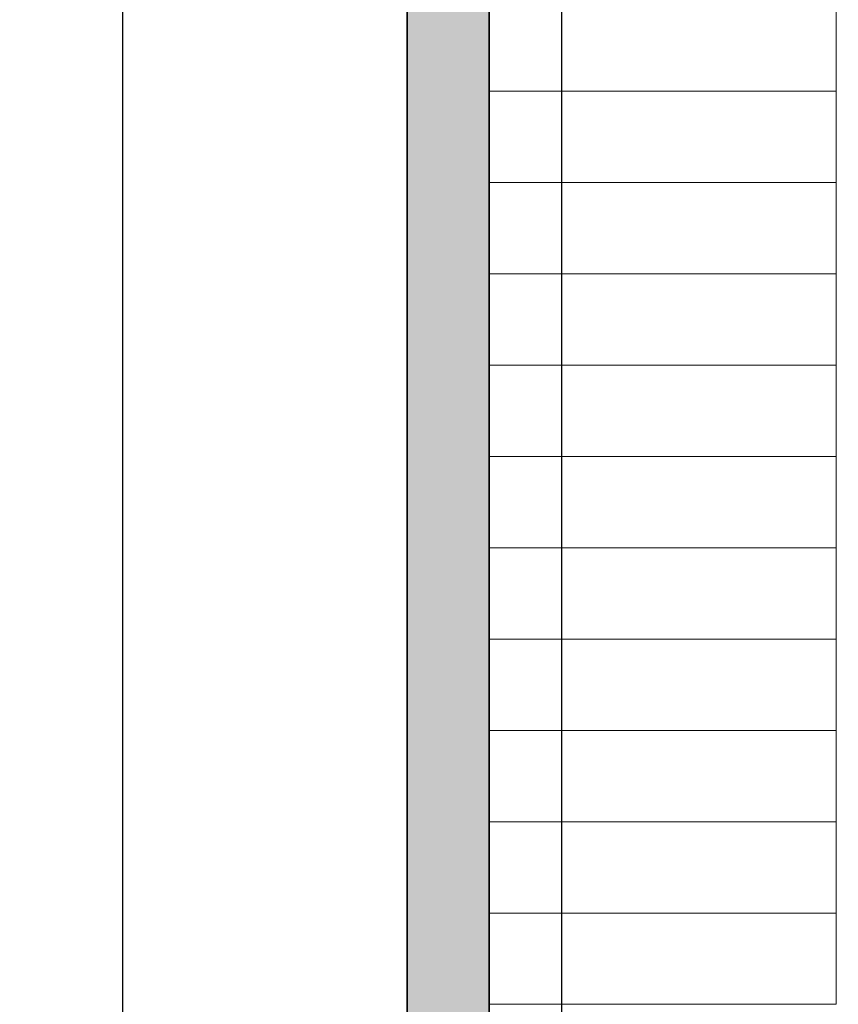
# Model space of a CAD drawing. Units: inches. Extents: x 37 to 706, y -568 to 110.
# Tile 2 of 24: x 37 to 126, y -450 to -342. Entities that reach past the tile are written whole.
import ezdxf

# ---------------------------------------------------------------- set-up
doc = ezdxf.new("R2010")
doc.units = ezdxf.units.IN
doc.header["$MEASUREMENT"] = 0
for name, color, linetype, lineweight in [('A-ANNO-DIMS', 2, 'Continuous', 18), ('A-FLOR-STRS', 7, 'Continuous', 18), ('A-WALL', 7, 'Continuous', 35), ('A-WALL-PATT', 252, 'Continuous', 13)]:
    doc.layers.add(name, color=color, linetype=linetype, lineweight=lineweight)
doc.styles.get("Standard").update_dxf_attribs({"font": 'arial.ttf'})
doc.dimstyles.get("Standard").update_dxf_attribs({"dimtxt": 0.18, "dimasz": 0.18, "dimexe": 0.18, "dimexo": 0.0625, "dimgap": 0.09, "dimtad": 0, "dimtih": 1, "dimtoh": 1, "dimdec": 0, "dimzin": 0, "dimdsep": 46, "dimlunit": 3, "dimtxsty": 'Standard', "dimcen": 0.09, "dimadec": 0, "dimazin": 0, "dimtfac": 1, "dimtdec": 0, "dimtofl": 0, "dimtmove": 0, "dimatfit": 3, "dimfxl": 1, "dimtolj": 1, "dimtzin": 0, "dimarcsym": 0})

# ---------------------------------------------------------------- blocks, each defined once
blk = doc.blocks.new('*D3')
at = {"layer": 'A-ANNO-DIMS', "color": 0, "lineweight": -2, "transparency": 16777216}
for p, q in [((78.9, 51.29), (47.67, 51.29)), ((47.85, 51.11), (47.85, -228.11)), ((47.85, -513.53), (47.85, -234.31)), ((78.9, -513.71), (47.67, -513.71))]:
    blk.add_line(p, q, dxfattribs=at)
at = {"layer": 'A-ANNO-DIMS', "color": 0, "transparency": 16777216}
for points in [[(47.82, 51.11), (47.88, 51.11), (47.85, 51.29)], [(47.82, -513.53), (47.88, -513.53), (47.85, -513.71)]]:
    blk.add_solid(points, dxfattribs=at)
at = {"layer": 'Defpoints', "color": 0, "transparency": 16777216}
for p in [(78.96, 51.29), (47.85, -513.71), (78.96, -513.71)]:
    blk.add_point(p, dxfattribs=at)
at = {"layer": 'A-ANNO-DIMS', "color": 0, "transparency": 16777216, "insert": (47.85, -231.21), "char_height": 6, "attachment_point": 5}
blk.add_mtext('\\A1;47\'-1"', dxfattribs=at)
blk = doc.blocks.new('*D54')
at = {"layer": 'A-ANNO-DIMS', "color": 0, "lineweight": -2, "transparency": 16777216}
for p, q in [((87.96, -303.77), (87.96, -567.64)), ((95.87, -303.77), (95.87, -567.64)), ((88.14, -567.46), (91.59, -567.46)), ((95.69, -567.46), (92.24, -567.46))]:
    blk.add_line(p, q, dxfattribs=at)
at = {"layer": 'A-ANNO-DIMS', "color": 0, "transparency": 16777216}
for points in [[(88.14, -567.43), (88.14, -567.49), (87.96, -567.46)], [(95.69, -567.43), (95.69, -567.49), (95.87, -567.46)]]:
    blk.add_solid(points, dxfattribs=at)
at = {"layer": 'Defpoints', "color": 0, "transparency": 16777216}
for p in [(87.96, -303.71), (95.87, -303.71), (95.87, -567.46)]:
    blk.add_point(p, dxfattribs=at)
at = {"layer": 'A-ANNO-DIMS', "color": 0, "transparency": 16777216, "insert": (91.91, -567.46), "char_height": 0.18, "attachment_point": 5}
blk.add_mtext('\\A1;0\'-8"', dxfattribs=at)

msp = doc.modelspace()

# ---------------------------------------------------------------- hatches: boundary and pattern name
at = {"layer": 'A-WALL-PATT'}
h = msp.add_hatch(color=256, dxfattribs=at)
h.dxf.hatch_style = 1
h.paths.add_polyline_path([(220.96, -351.71), (211.96, -351.71), (211.96, -513.71), (254.96, -513.71), (254.96, -504.71), (220.96, -504.71)], flags=17)
h.paths.add_polyline_path([(220.96, -294.71), (211.96, -294.71), (211.96, -303.71), (220.96, -303.71)], flags=17)
h.paths.add_polyline_path([(175.96, -294.71), (155.87, -294.71), (155.87, -303.71), (155.96, -303.71), (175.96, -303.71)], flags=17)
h.paths.add_polyline_path([(220.96, -16.71), (211.96, -16.71), (211.96, -142.71), (220.96, -142.71)], flags=17)
h.paths.add_polyline_path([(357.96, 51.29), (78.96, 51.29), (78.96, -513.71), (87.96, -513.71), (87.96, -303.71), (95.87, -303.71), (95.87, -294.71), (87.96, -294.71), (87.96, -142.71), (187.96, -142.71), (187.96, -133.71), (87.96, -133.71), (87.96, -25.71), (106.96, -25.71), (106.96, -16.71), (87.96, -16.71), (87.96, 42.29), (348.96, 42.29), (348.96, 17.13), (348.96, -133.71), (246.96, -133.71), (246.96, -142.71), (348.96, -142.71), (348.96, -294.71), (251.96, -294.71), (251.96, -303.71), (348.96, -303.71), (348.96, -351.71), (260.96, -351.71), (260.96, -329.71), (251.96, -329.71), (251.96, -360.71), (327.45, -360.71), (348.96, -360.71), (348.96, -504.71), (314.96, -504.71), (314.96, -513.71), (357.96, -513.71)])
h.paths.add_polyline_path([(416.96, -303.71), (402.96, -303.71), (402.96, -151.71), (478.96, -151.71), (478.96, -142.71), (402.96, -142.71), (402.96, -22.71), (409.96, -22.71), (409.96, -13.71), (402.96, -13.71), (402.96, 42.29), (663.96, 42.29), (663.96, -303.71), (566.96, -303.71), (566.96, -312.71), (663.96, -312.71), (663.96, -360.71), (575.96, -360.71), (575.96, -338.71), (566.96, -338.71), (566.96, -360.71), (566.96, -369.71), (642.45, -369.71), (663.96, -369.71), (663.96, -513.71), (629.96, -513.71), (629.96, -522.71), (672.96, -522.71), (672.96, 51.29), (393.96, 51.29), (393.96, -522.71), (402.96, -522.71), (402.96, -312.71), (416.96, -312.71)])
h.paths.add_polyline_path([(490.96, -303.71), (476.96, -303.71), (476.96, -312.71), (490.96, -312.71)], flags=17)
h.paths.add_polyline_path([(535.96, -303.71), (526.96, -303.71), (526.96, -312.71), (535.96, -312.71)], flags=17)
h.paths.add_polyline_path([(535.96, -369.71), (526.96, -369.71), (526.96, -522.71), (569.96, -522.71), (569.96, -513.71), (535.96, -513.71)], flags=17)
h.paths.add_polyline_path([(511.96, -13.71), (502.96, -13.71), (502.96, -151.71), (511.96, -151.71)], flags=17)
h.paths.add_polyline_path([(651.54, -142.71), (651.54, -120.18), (642.54, -120.18), (642.54, -142.71), (550.54, -142.71), (550.54, -120.71), (541.54, -120.71), (541.54, -142.71), (537.96, -142.71), (537.96, -151.71), (651.54, -151.71)], flags=17)
h.paths.add_polyline_path([(651.54, -85.71), (541.54, -85.71), (541.54, -94.71), (651.54, -94.71)], flags=17)
h.paths.add_polyline_path([(476.96, -13.71), (469.96, -13.71), (469.96, -22.71), (476.96, -22.71)], flags=17)
h.paths.add_polyline_path([(185.96, -16.71), (166.96, -16.71), (166.96, -25.71), (185.96, -25.71)], flags=17)
h.paths.add_polyline_path([(168.91, -414.72), (214.62, -414.72), (214.62, -392.33), (168.91, -392.33)], flags=25)

# ---------------------------------------------------------------- linework, layer by layer
at = {"layer": 'A-FLOR-STRS'}
for p, q in [((125.96, -339.71), (125.96, -449.71)), ((125.96, -349.71), (87.96, -349.71)), ((125.96, -359.71), (87.96, -359.71)), ((125.96, -369.71), (87.96, -369.71)), ((125.96, -379.71), (87.96, -379.71)), ((125.96, -389.71), (87.96, -389.71)), ((125.96, -399.71), (87.96, -399.71)), ((125.96, -409.71), (87.96, -409.71)), ((125.96, -419.71), (87.96, -419.71)), ((125.96, -429.71), (87.96, -429.71)), ((125.96, -439.71), (87.96, -439.71)), ((125.96, -449.71), (87.96, -449.71))]:
    msp.add_line(p, q, dxfattribs=at)
at = {"layer": 'A-WALL'}
for p, q in [((78.96, 51.29), (78.96, -513.71)), ((87.96, -303.71), (87.96, -513.71))]:
    msp.add_line(p, q, dxfattribs=at)

# ---------------------------------------------------------------- dimensions: what is measured, and where the dimension line sits
at = {"layer": 'A-ANNO-DIMS'}
dim = msp.add_linear_dim(base=(47.85, -513.71), p1=(78.96, 51.29), p2=(78.96, -513.71), angle=90, dimstyle='Standard', override={"dimtxt": 6, "dimclrd": 0, "dimclre": 0, "dimclrt": 0}, dxfattribs=at)
dim.commit()
dim.dimension.update_dxf_attribs({"geometry": '*D3', "text_midpoint": (47.85, -231.21)})
dim = msp.add_linear_dim(base=(95.87, -567.46), p1=(87.96, -303.71), p2=(95.87, -303.71), dimstyle='Standard', override={"dimdec": 1, "dimlfac": 1, "dimrnd": 0, "dimzin": 1, "dimdsep": 46, "dimlunit": 4, "dimfrac": 2}, dxfattribs=at)
dim.commit()
dim.dimension.update_dxf_attribs({"geometry": '*D54', "text_midpoint": (91.91, -567.46)})

doc.saveas('drawing.dxf')
